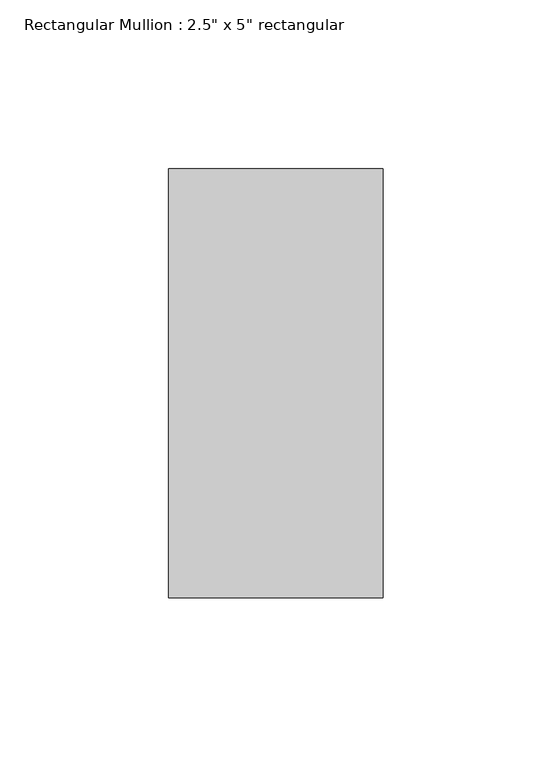
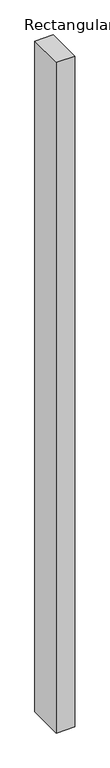
"""IFC4 building model written with IfcOpenShell, lengths in millimetres: member geometry."""

from ifc_helpers import new_model, si_unit, frame, origin, place, context, project, spatial, polyline, outline, extrude, source, transform, mapped, element, save


def member_2569944f(model_context):
    return source(origin(), model_context, "Body", "SweptSolid", [
        extrude(outline(polyline([(31.75, 63.5), (31.75, -63.5), (-31.75, -63.5), (-31.75, 63.5), (31.75, 63.5)])), frame((0.0, 0.0, -2432.05), z_axis=(0.0, 0.0, 1.0), x_axis=(1.0, 0.0, 0.0)), (0.0, 0.0, 1.0), 2432.05),
    ])


if __name__ == "__main__":
    model = new_model("IFC4")
    model_context = context("Model", 3, world=origin())
    ifc_project = project(units=[si_unit("LENGTHUNIT", "METRE", prefix="MILLI")], contexts=[model_context])
    site = spatial("IfcSite", under=ifc_project)
    building = spatial("IfcBuilding", under=site)
    placement = place(None, origin())
    member_shape = member_2569944f(model_context)
    element("IfcMember", 1, ObjectType="Rectangular Mullion : 2.5\" x 5\" rectangular", at=placement, inside=building, context=model_context, shape_type="MappedRepresentation", body=[
        mapped(member_shape, transform((0.0, 0.0, 0.0), x_axis=(1.0, 0.0, 0.0), y_axis=(0.0, 1.0, 0.0), z_axis=(0.0, 0.0, 1.0))),
    ])
    save(model, "model.ifc")

# Revit data of these elements
# Type "Rectangular Mullion : 2.5\" x 5\" rectangular"
#   built-in parameter 1007304 = 0.416667 (stored number, unit not read)
#   built-in parameter 1007301 = 0.104167 (stored number, unit not read)
#   built-in parameter 1007300 = 0.104167 (stored number, unit not read)
# Element 1 (IfcMember, "Rectangular Mullion : 2.5\" x 5\" rectangular")
#   Materials on its faces: "Aluminum"
# Materials
#   "Aluminum": class "Metal", colour RGB 247 247 247, transparency 0, Description = "Aluminum 6061", Cost = 0
